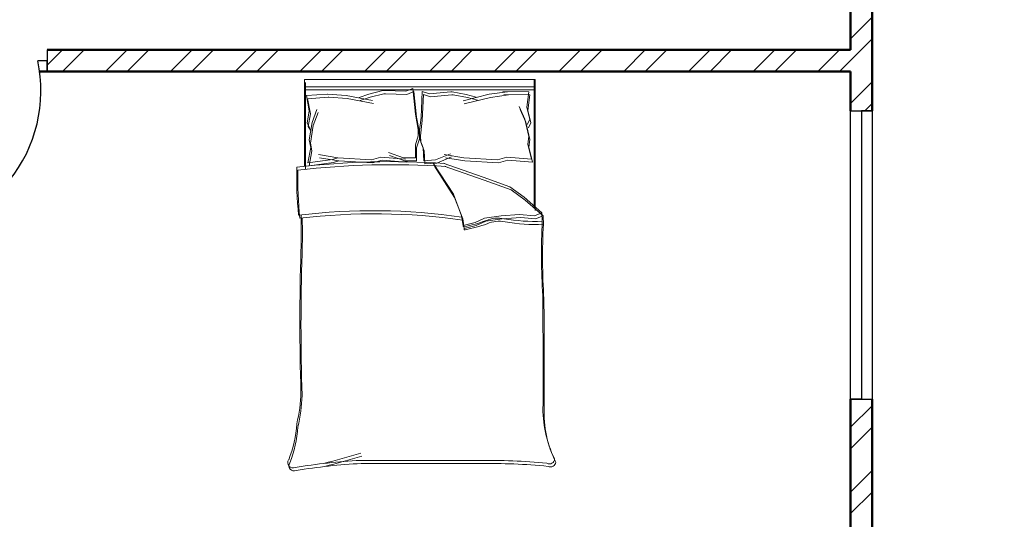
# Model space of a CAD drawing. Units: inches. Extents: x 963 to 2075, y 289 to 2657.
# Tile 88 of 98: x 1681 to 1885, y 2117 to 2221. Entities that reach past the tile are written whole.
import ezdxf

# ---------------------------------------------------------------- set-up
doc = ezdxf.new("R2010")
doc.units = ezdxf.units.IN
for name, color, linetype, lineweight in [('A-DOOR', 4, 'Continuous', 25), ('A-FURN', 8, 'Continuous', 18), ('A-GLAZ', 3, 'Continuous', 25), ('A-WALL', 7, 'Continuous', 50), ('A-WALL-PATT', 8, 'Continuous', 13)]:
    doc.layers.add(name, color=color, linetype=linetype, lineweight=lineweight)

# ---------------------------------------------------------------- blocks, each defined once
blk = doc.blocks.new('BED-DOUBLE')
for p, q in [((1236.12, 2450.52), (1254.23, 2450.52)), ((1236.12, 2450.52), (1254.23, 2450.52)), ((1236.76, 2450.75), (1254.87, 2450.75)), ((1236.76, 2450.75), (1254.87, 2450.75)), ((1237.61, 2444.71), (1236.89, 2449.81)), ((1236.89, 2449.81), (1240.07, 2449.23)), ((1237.61, 2444.71), (1236.89, 2449.81)), ((1236.89, 2449.81), (1240.07, 2449.23)), ((1238.25, 2444.94), (1237.53, 2450.04)), ((1237.53, 2450.04), (1240.71, 2449.46)), ((1238.25, 2444.94), (1237.53, 2450.04)), ((1237.53, 2450.04), (1240.71, 2449.46)), ((1245.13, 2449.96), (1244.12, 2449.38)), ((1245.13, 2449.96), (1244.12, 2449.38)), ((1245.77, 2450.18), (1244.76, 2449.61)), ((1245.77, 2450.18), (1244.76, 2449.61)), ((1247.74, 2449.52), (1245.13, 2449.96)), ((1247.74, 2449.52), (1245.13, 2449.96)), ((1248.37, 2449.75), (1245.77, 2450.18)), ((1248.37, 2449.75), (1245.77, 2450.18)), ((1250.92, 2450.1), (1247.74, 2449.52)), ((1250.92, 2450.1), (1247.74, 2449.52)), ((1251.56, 2450.33), (1248.37, 2449.75)), ((1251.56, 2450.33), (1248.37, 2449.75)), ((1250.89, 2450.1), (1251.22, 2445.82)), ((1250.89, 2450.1), (1251.22, 2445.82)), ((1251.53, 2450.32), (1251.86, 2446.04)), ((1251.53, 2450.32), (1251.86, 2446.04)), ((1252.7, 2450.52), (1252.7, 2402.73)), ((1252.7, 2450.52), (1252.7, 2402.73)), ((1253.34, 2450.75), (1253.34, 2402.96)), ((1253.34, 2450.75), (1253.34, 2402.96)), ((1254.87, 2450.75), (1254.87, 2402.73)), ((1239.24, 2447.84), (1238.58, 2443.81)), ((1239.24, 2447.84), (1238.58, 2443.81)), ((1240.07, 2449.23), (1241.66, 2449.52)), ((1240.07, 2449.23), (1241.66, 2449.52)), ((1240.71, 2449.46), (1242.3, 2449.75)), ((1240.71, 2449.46), (1242.3, 2449.75)), ((1241.66, 2449.52), (1245.28, 2448.94)), ((1241.66, 2449.52), (1245.28, 2448.94)), ((1242.3, 2449.75), (1245.92, 2449.17)), ((1242.3, 2449.75), (1245.92, 2449.17)), ((1245.28, 2448.94), (1248.02, 2447.93)), ((1245.28, 2448.94), (1248.02, 2447.93)), ((1245.92, 2449.17), (1248.66, 2448.16)), ((1245.92, 2449.17), (1248.66, 2448.16)), ((1238.6, 2447.61), (1237.94, 2443.58)), ((1238.6, 2447.61), (1237.94, 2443.58)), ((1251.21, 2445.71), (1250.92, 2441.89)), ((1251.21, 2445.71), (1250.92, 2441.89)), ((1251.22, 2445.82), (1251.21, 2445.71)), ((1251.22, 2445.82), (1251.21, 2445.71)), ((1251.84, 2445.94), (1251.56, 2442.11)), ((1251.84, 2445.94), (1251.56, 2442.11)), ((1251.86, 2446.04), (1251.84, 2445.94)), ((1251.86, 2446.04), (1251.84, 2445.94)), ((1237.94, 2443.58), (1237.61, 2444.71)), ((1237.94, 2443.58), (1237.61, 2444.71)), ((1238.58, 2443.81), (1238.15, 2436.8)), ((1238.58, 2443.81), (1238.15, 2436.8)), ((1238.58, 2443.81), (1238.25, 2444.94)), ((1238.58, 2443.81), (1238.25, 2444.94)), ((1237.94, 2443.58), (1237.51, 2436.57)), ((1237.94, 2443.58), (1237.51, 2436.57)), ((1250.92, 2441.89), (1249.9, 2436.39)), ((1250.92, 2441.89), (1249.9, 2436.39)), ((1251.56, 2442.11), (1250.54, 2436.62)), ((1251.56, 2442.11), (1250.54, 2436.62)), ((1174.99, 2438.93), (1174.99, 2414.32)), ((1174.99, 2438.93), (1174.99, 2414.32)), ((1175.63, 2439.16), (1175.63, 2414.55)), ((1175.63, 2439.16), (1175.63, 2414.55)), ((1250.48, 2439.14), (1251.21, 2437.12)), ((1250.48, 2439.14), (1251.21, 2437.12)), ((1251.12, 2439.37), (1251.84, 2437.34)), ((1251.12, 2439.37), (1251.84, 2437.34)), ((1237.51, 2436.57), (1238.06, 2434.61)), ((1237.51, 2436.57), (1238.06, 2434.61)), ((1238.15, 2436.8), (1238.7, 2434.84)), ((1238.15, 2436.8), (1238.7, 2434.84)), ((1251.21, 2437.12), (1251.93, 2434.22)), ((1251.21, 2437.12), (1251.93, 2434.23)), ((1251.84, 2437.34), (1252.57, 2434.45)), ((1251.84, 2437.34), (1252.57, 2434.45)), ((1238.06, 2434.61), (1237.66, 2429.48)), ((1238.06, 2434.61), (1237.66, 2429.48)), ((1238.7, 2434.84), (1238.3, 2429.71)), ((1238.7, 2434.84), (1238.3, 2429.71)), ((1251.93, 2433.9), (1251.78, 2429.46)), ((1251.93, 2433.9), (1251.78, 2429.46)), ((1251.93, 2434.23), (1251.93, 2433.9)), ((1251.93, 2434.22), (1251.93, 2433.9)), ((1252.57, 2434.13), (1252.42, 2429.69)), ((1252.57, 2434.13), (1252.42, 2429.69)), ((1252.57, 2434.45), (1252.57, 2434.13)), ((1252.57, 2434.45), (1252.57, 2434.13)), ((1237.97, 2429.89), (1239.06, 2433.04)), ((1237.97, 2429.89), (1239.06, 2433.04)), ((1238.61, 2430.12), (1239.7, 2433.26)), ((1238.61, 2430.12), (1239.7, 2433.26)), ((1237.97, 2427.43), (1237.97, 2429.89)), ((1237.97, 2427.43), (1237.97, 2429.89)), ((1238.61, 2427.66), (1238.61, 2430.12)), ((1238.61, 2427.66), (1238.61, 2430.12)), ((1251.78, 2429.46), (1252.36, 2428.01)), ((1251.78, 2429.46), (1252.36, 2428.01)), ((1252.42, 2429.69), (1253, 2428.24)), ((1252.42, 2429.69), (1253, 2428.24)), ((1240.65, 2427.43), (1237.97, 2427.43)), ((1240.65, 2427.43), (1237.97, 2427.43)), ((1241.29, 2427.66), (1238.61, 2427.66)), ((1241.29, 2427.66), (1238.61, 2427.66)), ((1242.53, 2426.86), (1240.65, 2427.43)), ((1242.53, 2426.86), (1240.65, 2427.43)), ((1243.17, 2427.08), (1241.29, 2427.66)), ((1243.17, 2427.08), (1241.29, 2427.66)), ((1247.01, 2427.43), (1243.83, 2426.86)), ((1247.01, 2427.43), (1243.83, 2426.86)), ((1247.65, 2427.66), (1244.47, 2427.08)), ((1247.65, 2427.66), (1244.47, 2427.08)), ((1252.36, 2428.01), (1247.01, 2427.43)), ((1252.36, 2428.01), (1247.01, 2427.43)), ((1253, 2428.24), (1247.65, 2427.66)), ((1253, 2428.24), (1247.65, 2427.66)), ((1240.02, 2425.86), (1237.34, 2425.7)), ((1240.02, 2425.86), (1237.34, 2425.7)), ((1237.34, 2425.7), (1237.49, 2423.24)), ((1237.34, 2425.7), (1237.49, 2423.24)), ((1240.66, 2426.09), (1237.98, 2425.93)), ((1240.66, 2426.09), (1237.98, 2425.93)), ((1237.98, 2425.93), (1238.13, 2423.47)), ((1237.98, 2425.93), (1238.13, 2423.47)), ((1241.86, 2426.56), (1240.02, 2425.86)), ((1241.86, 2426.56), (1240.02, 2425.86)), ((1242.49, 2426.79), (1240.66, 2426.09)), ((1242.49, 2426.79), (1240.66, 2426.09)), ((1243.15, 2426.64), (1241.86, 2426.56)), ((1243.15, 2426.64), (1241.86, 2426.56)), ((1243.79, 2426.87), (1242.49, 2426.79)), ((1243.79, 2426.87), (1242.49, 2426.79)), ((1243.83, 2426.86), (1242.53, 2426.86)), ((1243.83, 2426.86), (1242.53, 2426.86)), ((1246.37, 2426.26), (1243.15, 2426.64)), ((1246.37, 2426.26), (1243.15, 2426.64)), ((1244.47, 2427.08), (1243.17, 2427.08)), ((1244.47, 2427.08), (1243.17, 2427.08)), ((1247, 2426.49), (1243.79, 2426.87)), ((1247, 2426.49), (1243.79, 2426.87)), ((1251.74, 2426.02), (1246.37, 2426.26)), ((1251.74, 2426.02), (1246.37, 2426.26)), ((1252.38, 2426.25), (1247, 2426.49)), ((1252.38, 2426.25), (1247, 2426.49)), ((1251.25, 2424.54), (1251.74, 2426.02)), ((1251.25, 2424.54), (1251.74, 2426.02)), ((1251.89, 2424.77), (1252.38, 2426.25)), ((1251.89, 2424.77), (1252.38, 2426.25)), ((1236.85, 2423.74), (1230.36, 2419.55)), ((1236.85, 2423.74), (1230.36, 2419.55)), ((1237.49, 2423.96), (1231, 2419.77)), ((1237.49, 2423.96), (1231, 2419.77)), ((1237.49, 2423.24), (1238.78, 2420.17)), ((1237.49, 2423.24), (1238.78, 2420.17)), ((1238.13, 2423.47), (1239.42, 2420.4)), ((1238.13, 2423.47), (1239.42, 2420.4)), ((1251.68, 2420.11), (1251.25, 2424.54)), ((1251.68, 2420.11), (1251.25, 2424.54)), ((1252.31, 2420.34), (1251.89, 2424.77)), ((1252.31, 2420.34), (1251.89, 2424.77)), ((1233.92, 2413.35), (1236.85, 2421.69)), ((1233.92, 2413.35), (1236.85, 2421.69)), ((1234.56, 2413.58), (1237.49, 2421.92)), ((1234.56, 2413.58), (1237.49, 2421.92)), ((1238.6, 2421.43), (1237.94, 2417.4)), ((1238.6, 2421.43), (1237.94, 2417.4)), ((1239.24, 2421.66), (1238.58, 2417.63)), ((1239.24, 2421.66), (1238.58, 2417.63)), ((1230.36, 2419.55), (1225.87, 2417.84)), ((1230.36, 2419.55), (1225.87, 2417.84)), ((1231, 2419.77), (1226.51, 2418.07)), ((1231, 2419.77), (1226.51, 2418.07)), ((1251.15, 2416.86), (1251.7, 2419.79)), ((1251.15, 2416.86), (1251.7, 2419.79)), ((1251.7, 2419.79), (1251.68, 2420.11)), ((1251.7, 2419.79), (1251.68, 2420.11)), ((1251.79, 2417.09), (1252.33, 2420.02)), ((1251.79, 2417.09), (1252.33, 2420.02)), ((1252.33, 2420.02), (1252.31, 2420.34)), ((1252.33, 2420.02), (1252.31, 2420.34)), ((1225.87, 2417.84), (1223.86, 2417.53)), ((1225.87, 2417.84), (1223.86, 2417.53)), ((1223.86, 2417.53), (1224.47, 2415.05)), ((1223.86, 2417.53), (1224.47, 2415.05)), ((1226.51, 2418.07), (1224.49, 2417.76)), ((1226.51, 2418.07), (1224.49, 2417.76)), ((1224.49, 2417.76), (1225.11, 2415.28)), ((1224.49, 2417.76), (1225.11, 2415.28)), ((1237.94, 2417.4), (1237.51, 2410.39)), ((1237.94, 2417.4), (1237.51, 2410.39)), ((1238.58, 2417.63), (1238.15, 2410.62)), ((1238.58, 2417.63), (1238.15, 2410.62)), ((1251.16, 2412.08), (1249.81, 2417.5)), ((1251.16, 2412.08), (1249.81, 2417.5)), ((1251.8, 2412.31), (1250.45, 2417.73)), ((1251.8, 2412.31), (1250.45, 2417.73)), ((1251.2, 2415.02), (1251.79, 2417.09)), ((1251.2, 2415.02), (1251.79, 2417.09)), ((1224.47, 2415.05), (1225.4, 2413.04)), ((1224.47, 2415.05), (1225.4, 2413.04)), ((1225.11, 2415.28), (1226.04, 2413.27)), ((1225.11, 2415.28), (1226.04, 2413.27)), ((1250.56, 2414.79), (1251.15, 2416.86)), ((1250.56, 2414.79), (1251.15, 2416.86)), ((1225.4, 2413.04), (1225.87, 2409.63)), ((1225.4, 2413.04), (1225.87, 2409.63)), ((1226.04, 2413.27), (1226.51, 2409.86)), ((1226.04, 2413.27), (1226.51, 2409.86)), ((1231.9, 2407.77), (1233.92, 2413.35)), ((1231.9, 2407.78), (1233.92, 2413.35)), ((1232.54, 2408), (1234.56, 2413.58)), ((1232.54, 2408), (1234.56, 2413.58)), ((1251.69, 2408.28), (1251.16, 2412.08)), ((1251.69, 2408.28), (1251.16, 2412.08)), ((1252.33, 2408.51), (1251.8, 2412.31)), ((1252.33, 2408.51), (1251.8, 2412.31)), ((1225.87, 2409.63), (1226.18, 2405.76)), ((1225.87, 2409.63), (1226.18, 2405.76)), ((1226.51, 2409.86), (1226.82, 2405.99)), ((1226.51, 2409.86), (1226.82, 2405.99)), ((1237.51, 2410.39), (1238.06, 2408.43)), ((1237.51, 2410.39), (1238.06, 2408.43)), ((1238.15, 2410.62), (1238.7, 2408.66)), ((1238.15, 2410.62), (1238.7, 2408.66)), ((1251.68, 2403.88), (1251.77, 2409.29)), ((1251.68, 2403.88), (1251.77, 2409.28)), ((1251.77, 2409.29), (1251.69, 2408.28)), ((1251.77, 2409.28), (1251.69, 2408.28)), ((1252.31, 2404.11), (1252.41, 2409.51)), ((1252.31, 2404.11), (1252.41, 2409.51)), ((1252.41, 2409.51), (1252.33, 2408.51)), ((1252.41, 2409.51), (1252.33, 2408.51)), ((1229.74, 2404.83), (1231.9, 2407.78)), ((1229.74, 2404.83), (1231.9, 2407.77)), ((1230.38, 2405.06), (1232.54, 2408)), ((1230.38, 2405.06), (1232.54, 2408)), ((1238.06, 2408.43), (1237.66, 2403.3)), ((1238.06, 2408.43), (1237.66, 2403.3)), ((1238.7, 2408.66), (1238.3, 2403.52)), ((1238.7, 2408.66), (1238.3, 2403.52)), ((1226.18, 2405.76), (1225.87, 2402.66)), ((1226.18, 2405.76), (1225.87, 2402.66)), ((1226.49, 2401.13), (1229.74, 2404.83)), ((1226.49, 2401.13), (1229.74, 2404.83)), ((1226.82, 2405.99), (1226.51, 2402.89)), ((1226.82, 2405.99), (1226.51, 2402.89)), ((1227.13, 2401.36), (1230.38, 2405.06)), ((1227.13, 2401.36), (1230.38, 2405.06)), ((1243.04, 2404.11), (1246.61, 2404.91)), ((1243.04, 2404.11), (1246.61, 2404.91)), ((1245.98, 2404.69), (1248.65, 2405.87)), ((1245.98, 2404.69), (1248.65, 2405.87)), ((1246.61, 2404.91), (1249.29, 2406.1)), ((1246.61, 2404.91), (1249.29, 2406.09)), ((1225.87, 2402.66), (1226.49, 2401.13)), ((1225.87, 2402.66), (1226.49, 2401.13)), ((1226.51, 2402.89), (1227.13, 2401.36)), ((1226.51, 2402.89), (1227.13, 2401.36)), ((1254.23, 2402.73), (1227.62, 2402.73)), ((1254.23, 2402.73), (1227.62, 2402.73)), ((1254.87, 2402.96), (1228.26, 2402.96)), ((1254.87, 2402.96), (1228.26, 2402.96)), ((1237.66, 2403.3), (1240.8, 2404.07)), ((1237.66, 2403.3), (1240.8, 2404.07)), ((1238.3, 2403.52), (1241.44, 2404.3)), ((1238.3, 2403.52), (1241.44, 2404.3)), ((1240.8, 2404.07), (1242.4, 2403.88)), ((1240.8, 2404.07), (1242.4, 2403.88)), ((1241.44, 2404.3), (1243.04, 2404.11)), ((1241.44, 2404.3), (1243.04, 2404.11)), ((1242.4, 2403.88), (1245.98, 2404.69)), ((1242.4, 2403.88), (1245.98, 2404.69)), ((1245.89, 2403.67), (1244.85, 2404.18)), ((1245.89, 2403.67), (1244.85, 2404.18)), ((1246.53, 2403.89), (1245.49, 2404.41)), ((1246.53, 2403.89), (1245.49, 2404.41)), ((1248.46, 2404.26), (1245.89, 2403.67)), ((1248.46, 2404.26), (1245.89, 2403.67)), ((1249.1, 2404.49), (1246.53, 2403.89)), ((1249.1, 2404.49), (1246.53, 2403.89)), ((1251.68, 2403.88), (1248.46, 2404.26)), ((1251.68, 2403.88), (1248.46, 2404.26)), ((1252.31, 2404.11), (1249.1, 2404.49)), ((1252.31, 2404.11), (1249.1, 2404.49)), ((1254.87, 2402.73), (1254.23, 2402.73)), ((1224.74, 2401.05), (1226.49, 2401.13, 3.87)), ((1224.74, 2401.05), (1226.49, 2401.13, 3.87)), ((1225.38, 2401.28), (1227.13, 2401.36, 3.87)), ((1225.38, 2401.28), (1227.13, 2401.36, 3.87))]:
    blk.add_line(p, q)
for centre, radius, start, end in [((1174.51, 2452.91), 1.09, 56.1736, 203.4781), ((1174.51, 2452.91), 1.09, 56.1736, 203.4781), ((1175.15, 2453.14), 1.09, 56.1736, 203.4781), ((1175.15, 2453.14), 1.09, 56.1736, 203.4781), ((1184.6, 2475.88), 23.56, 247.9751, 266.652), ((1184.6, 2475.88), 23.56, 247.9751, 266.652), ((1053.4, 2432.57), 121.76, 2.9958, 9.4091), ((1053.4, 2432.57), 121.76, 2.9958, 9.4091), ((1054.03, 2432.8), 121.76, 2.9958, 9.4091), ((1054.03, 2432.8), 121.76, 2.9958, 9.4091), ((1183.96, 2475.65), 23.56, 247.9751, 266.652), ((1183.96, 2475.65), 23.56, 247.9751, 266.652), ((1189.72, 2480.89), 29.63, 256.0648, 268.9113), ((1189.72, 2480.89), 29.63, 256.0648, 268.9113), ((1190.36, 2481.12), 29.63, 256.0648, 268.9113), ((1190.36, 2481.12), 29.63, 256.0648, 268.9113), ((1234.14, 2368.83), 83.31, 88.7218, 95.604), ((1234.14, 2368.83), 83.31, 88.7218, 95.604), ((1098.56, 2436.47), 129.02, 351.7845, 6.9006), ((1098.56, 2436.47), 129.02, 351.7845, 6.9006), ((1234.78, 2369.06), 83.31, 88.7218, 95.604), ((1234.78, 2369.06), 83.31, 88.7218, 95.604), ((1072.18, 2432.64), 164.97, 356.0865, 6.7821), ((1072.18, 2432.64), 164.97, 356.0865, 6.7821), ((1072.82, 2432.86), 164.97, 356.0865, 6.7821), ((1072.82, 2432.86), 164.97, 356.0865, 6.7821), ((1203.62, 1969.17), 482.31, 88.2277, 91.7185), ((1203.62, 1969.17), 482.31, 88.2277, 91.7185), ((1204.26, 1969.4), 482.31, 88.2277, 91.7185), ((1204.26, 1969.4), 482.31, 88.2277, 91.7185), ((1223.06, 2621.3), 170.11, 268.4762, 271.0082), ((1223.06, 2621.3), 170.11, 268.4762, 271.0082), ((1223.7, 2621.53), 170.11, 268.4762, 271.0082), ((1223.7, 2621.53), 170.11, 268.4762, 271.0082), ((1097.92, 2436.24), 129.02, 351.7845, 6.9006), ((1097.92, 2436.24), 129.02, 351.7845, 6.9006), ((1277.94, 2471.22), 106.46, 193.3832, 197.7053), ((1277.94, 2471.22), 106.46, 193.3832, 197.7053), ((1278.58, 2471.44), 106.46, 193.3832, 197.7053), ((1278.58, 2471.44), 106.46, 193.3832, 197.7053), ((1223.79, 2417.36), 0.185, 70.2464, 181.1377), ((1223.79, 2417.36), 0.185, 70.2464, 181.1377), ((1252.75, 2422.84), 29.65, 190.6617, 199.8806), ((1252.75, 2422.84), 29.65, 190.6617, 199.8806), ((1224.43, 2417.59), 0.185, 70.2464, 181.1377), ((1224.43, 2417.59), 0.185, 70.2464, 181.1377), ((1253.39, 2423.07), 29.65, 190.6617, 199.8806), ((1253.39, 2423.07), 29.65, 190.6617, 199.8806), ((1041.96, 2412.84), 133.04, 354.4998, 0.6351), ((1041.96, 2412.84), 133.04, 354.4998, 0.6351), ((1042.6, 2413.07), 133.04, 354.4998, 0.6351), ((1042.6, 2413.07), 133.04, 354.4998, 0.6351), ((1219.81, 2410.48), 6.22, 348.6608, 23.7384), ((1219.81, 2410.48), 6.22, 348.6608, 23.7384), ((1219.17, 2410.25), 6.22, 348.6608, 23.7384), ((1219.17, 2410.25), 6.22, 348.6608, 23.7384), ((1260.89, 2402.67), 36.18, 169.8763, 182.5657), ((1260.89, 2402.67), 36.18, 169.8763, 182.5657), ((1261.53, 2402.9), 36.18, 169.8763, 182.5657), ((1261.53, 2402.9), 36.18, 169.8763, 182.5657), ((1185.57, 2377.84), 23.07, 87.4714, 116.4681), ((1185.57, 2377.84), 23.07, 87.4714, 116.4681), ((1186.21, 2378.07), 23.07, 87.4714, 116.4681), ((1186.21, 2378.07), 23.07, 87.4714, 116.4681), ((1186.41, 6962.74), 4561.86, 270.00217, 270.28689), ((1186.41, 6962.74), 4561.86, 270.00217, 270.28689), ((1187.05, 6962.97), 4561.86, 270.00217, 270.28689), ((1187.05, 6962.97), 4561.86, 270.00217, 270.28689), ((1217.92, 2271.73), 129.5, 86.9791, 93.8365), ((1217.92, 2271.73), 129.5, 86.9791, 93.8365), ((1218.56, 2271.96), 129.5, 86.9791, 93.8365), ((1218.56, 2271.96), 129.5, 86.9791, 93.8365), ((1175.36, 2399.58), 1.1, 152.6588, 266.02), ((1175.36, 2399.58), 1.1, 152.6588, 266.02), ((1176, 2399.81), 1.1, 152.6588, 266.02), ((1176, 2399.81), 1.1, 152.6588, 266.02)]:
    blk.add_arc(centre, radius, start, end)

msp = doc.modelspace()

# ---------------------------------------------------------------- hatches: boundary and pattern name
at = {"layer": 'A-WALL-PATT'}
h = msp.add_hatch(dxfattribs=at)
h.set_pattern_fill('ANSI32', color=256)
h.paths.add_polyline_path([(1296.92, 2558.32), (1203.92, 2558.32), (1203.92, 2493.82), (1191.53, 2493.82), (1191.53, 2489.32), (1211.06, 2489.32), (1211.06, 2492.02), (1211.06, 2493.82), (1208.42, 2493.82), (1208.42, 2553.82), (1292.42, 2553.82), (1292.42, 2538.86), (1296.92, 2538.86)])
h.paths.add_polyline_path([(1442.42, 2558.32), (1349.42, 2558.32), (1349.42, 2538.94), (1353.92, 2538.94), (1353.92, 2553.82), (1437.92, 2553.82), (1437.92, 2493.82), (1434.54, 2493.82), (1434.54, 2489.32), (1448.31, 2489.32), (1448.31, 2491.57), (1448.31, 2493.82), (1442.42, 2493.82)])
h.paths.add_polyline_path([(1415.55, 2491.57), (1415.55, 2493.82), (1340.94, 2493.82), (1340.94, 2489.32), (1371.92, 2489.32), (1371.92, 2378.32), (1367.6, 2378.32), (1367.6, 2373.82), (1371.92, 2373.82), (1371.92, 2355.19), (1376.42, 2355.19), (1376.42, 2489.32), (1415.55, 2489.32)])
h.paths.add_polyline_path([(1304.94, 2491.57), (1304.94, 2493.82), (1296.92, 2493.82), (1296.92, 2514.86), (1292.42, 2514.86), (1292.42, 2493.82), (1232.81, 2493.82), (1232.81, 2489.32), (1256.42, 2489.32), (1256.42, 2327.32), (1253.71, 2327.32), (1253.71, 2322.82), (1328.42, 2322.82), (1328.42, 2331.15), (1323.92, 2331.15), (1323.92, 2327.32), (1260.92, 2327.32), (1260.92, 2373.82), (1323.92, 2373.82), (1323.92, 2357.81), (1328.42, 2357.81), (1328.42, 2373.82), (1346.01, 2373.82), (1346.01, 2376.07), (1346.01, 2378.32), (1260.92, 2378.32), (1260.92, 2489.32), (1304.94, 2489.32)])
h.paths.add_polyline_path([(1226.65, 2327.32), (1124.42, 2327.32), (1124.42, 2347.45), (1119.92, 2347.45), (1119.92, 2322.82), (1163.42, 2322.82), (1163.42, 2305.43), (1165.67, 2305.43), (1167.92, 2305.43), (1167.92, 2322.82), (1226.65, 2322.82), (1226.65, 2325.07)])
h.paths.add_polyline_path([(1095.92, 2489.32), (1124.42, 2489.32), (1131.53, 2489.32), (1131.53, 2491.57), (1131.53, 2493.82), (1119.92, 2493.82), (1091.42, 2493.82), (1091.42, 2417.32), (1095.92, 2417.32), (1119.92, 2417.32), (1119.92, 2407.45), (1124.42, 2407.45), (1124.42, 2421.82), (1095.92, 2421.82)])
h.paths.add_polyline_path([(1512.92, 2558.32), (1508.42, 2558.32), (1508.42, 2493.82), (1503.4, 2493.82), (1503.4, 2489.32), (1508.42, 2489.32), (1508.42, 2327.32), (1376.42, 2327.32), (1376.42, 2330.27), (1371.92, 2330.27), (1371.92, 2298.74), (1376.42, 2298.74), (1376.42, 2322.82), (1508.42, 2322.82), (1508.42, 2165.32), (1504.26, 2165.32), (1504.26, 2160.82), (1508.42, 2160.82), (1508.42, 2108.32), (1512.92, 2108.32), (1512.92, 2160.82), (1516.18, 2160.82), (1516.18, 2163.07), (1516.18, 2165.32), (1512.92, 2165.32), (1512.92, 2322.82), (1644.92, 2322.82), (1644.92, 2298.74), (1649.42, 2298.74), (1649.42, 2322.82), (1649.42, 2330.94), (1647.17, 2330.94), (1644.92, 2330.94), (1644.92, 2327.32), (1512.92, 2327.32), (1512.92, 2489.32), (1516.76, 2489.32), (1516.76, 2491.57), (1516.76, 2493.82), (1512.92, 2493.82)])
h.paths.add_polyline_path([(1671.92, 2558.32), (1578.92, 2558.32), (1578.92, 2493.82), (1573.53, 2493.82), (1573.53, 2489.32), (1586.54, 2489.32), (1586.54, 2491.57), (1586.54, 2493.82), (1583.42, 2493.82), (1583.42, 2553.82), (1667.42, 2553.82), (1667.42, 2541.11), (1671.92, 2541.11)])
h.paths.add_polyline_path([(1681.26, 2493.82), (1671.92, 2493.82), (1671.92, 2517.11), (1667.42, 2517.11), (1667.42, 2493.82), (1610.22, 2493.82), (1610.22, 2489.32), (1644.92, 2489.32), (1644.92, 2357.87), (1649.42, 2357.87), (1649.42, 2373.82), (1652.2, 2373.82), (1652.2, 2375.83), (1652.2, 2378.32), (1649.42, 2378.32), (1649.42, 2489.32), (1681.26, 2489.32), (1681.26, 2491.57)])
h.paths.add_polyline_path([(1821.92, 2558.32), (1728.92, 2558.32), (1728.92, 2541), (1733.42, 2541), (1733.42, 2553.82), (1817.42, 2553.82), (1817.42, 2493.82), (1813.51, 2493.82), (1813.51, 2489.32), (1830.08, 2489.32), (1830.08, 2491.57), (1830.08, 2493.82), (1821.92, 2493.82)])
h.paths.add_polyline_path([(1794.24, 2493.82), (1717.26, 2493.82), (1717.26, 2489.32), (1760.42, 2489.32), (1760.42, 2378.32), (1674.4, 2378.32), (1674.4, 2373.82), (1692.92, 2373.82), (1692.92, 2356.95), (1697.42, 2356.95), (1697.42, 2373.82), (1760.42, 2373.82), (1760.42, 2327.32), (1697.42, 2327.32), (1697.42, 2333.34), (1692.92, 2333.34), (1692.92, 2322.82), (1768.04, 2322.82), (1768.04, 2325.07), (1768.04, 2327.32), (1764.92, 2327.32), (1764.92, 2489.32), (1794.24, 2489.32)])
h.paths.add_polyline_path([(1733.42, 2517), (1728.92, 2517), (1728.92, 2493.82), (1733.42, 2493.82)], flags=17)
h.paths.add_polyline_path([(1929.92, 2493.82), (1890.08, 2493.82), (1890.08, 2489.32), (1896.92, 2489.32), (1925.42, 2489.32), (1925.42, 2421.82), (1896.92, 2421.82), (1896.92, 2408.32), (1901.42, 2408.32), (1901.42, 2417.32), (1925.42, 2417.32), (1929.92, 2417.32)])
h.paths.add_polyline_path([(1901.42, 2348.32), (1896.92, 2348.32), (1896.92, 2327.32), (1800.42, 2327.32), (1800.42, 2322.82), (1853.42, 2322.82), (1853.42, 2309.45), (1857.92, 2309.45), (1857.92, 2322.82), (1901.42, 2322.82)])
h.paths.add_polyline_path([(1857.92, 2249.45), (1853.42, 2249.45), (1853.42, 2214.82), (1686.31, 2214.82), (1686.31, 2210.32), (1853.42, 2210.32), (1853.42, 2202.13), (1857.92, 2202.13), (1857.92, 2210.32)])
h.paths.add_polyline_path([(1857.92, 2142.13), (1853.42, 2142.13), (1853.42, 2115.42), (1841.42, 2115.42), (1841.42, 2088.53), (1841.42, 2046.95), (1845.92, 2046.95), (1845.92, 2110.92), (1905.92, 2110.92), (1905.92, 2092.52), (1910.42, 2092.52), (1910.42, 2115.42), (1857.92, 2115.42)])
h.paths.add_polyline_path([(1532.44, 1482.34), (1573.46, 1482.34), (1573.46, 1501), (1532.44, 1501)], flags=9)
h.paths.add_polyline_path([(1438.66, 1486.3), (1479.68, 1486.3), (1479.68, 1504.96), (1438.66, 1504.96)], flags=9)
h.paths.add_polyline_path([(1411.22, 1365.31), (1659.14, 1365.31), (1659.14, 1402.4), (1411.22, 1402.4)], flags=9)
h.paths.add_polyline_path([(1185.67, 2296.3), (1248.16, 2296.3), (1248.16, 2314.95), (1185.67, 2314.95)], flags=9)
h.paths.add_polyline_path([(1177.31, 2187.35), (1216.15, 2187.35), (1216.15, 2206.01), (1177.31, 2206.01)], flags=9)
h.paths.add_polyline_path([(1295.1, 1602.08), (1328.26, 1602.08), (1328.26, 1620.74), (1295.1, 1620.74)], flags=9)
h.paths.add_polyline_path([(1525.13, 2005.99), (1558.39, 2005.99), (1558.39, 2024.65), (1525.13, 2024.65)], flags=9)
h.paths.add_polyline_path([(1459.61, 1977.13), (1472.19, 1977.13), (1472.19, 1987.43), (1459.61, 1987.43)], flags=9)
h.paths.add_polyline_path([(1467.81, 2053.68), (1480.02, 2053.68), (1480.02, 2063.98), (1467.81, 2063.98)], flags=9)
h.paths.add_polyline_path([(1555.18, 2119.02), (1584.56, 2119.02), (1584.56, 2137.68), (1555.18, 2137.68)], flags=25)
h.paths.add_polyline_path([(1405.39, 2115.29), (1444.48, 2115.29), (1444.48, 2133.95), (1405.39, 2133.95)], flags=25)
h.paths.add_polyline_path([(1698.48, 2004.26), (1727.69, 2004.26), (1727.69, 2022.92), (1698.48, 2022.92)], flags=9)
h.paths.add_polyline_path([(1612.16, 1972.86), (1629.02, 1972.86), (1629.02, 1983.16), (1612.16, 1983.16)], flags=9)
h.paths.add_polyline_path([(1608.29, 2060.04), (1625.15, 2060.04), (1625.15, 2070.34), (1608.29, 2070.34)], flags=9)
h.paths.add_polyline_path([(1527.95, 1684.4), (1566.79, 1684.4), (1566.79, 1703.06), (1527.95, 1703.06)], flags=9)
h.paths.add_polyline_path([(1422.79, 1683.59), (1461.63, 1683.59), (1461.63, 1702.25), (1422.79, 1702.25)], flags=9)
h.paths.add_polyline_path([(1531.26, 1732.46), (1574.01, 1732.46), (1574.01, 1751.12), (1531.26, 1751.12)], flags=9)
h.paths.add_polyline_path([(1402.87, 1732.85), (1439.8, 1732.85), (1439.8, 1751.5), (1402.87, 1751.5)], flags=9)
h.paths.add_polyline_path([(1243.12, 1923.13), (1281.96, 1923.13), (1281.96, 1941.79), (1243.12, 1941.79)], flags=9)
h.paths.add_polyline_path([(1181.75, 1792.27), (1244.24, 1792.27), (1244.24, 1810.93), (1181.75, 1810.93)], flags=9)
h.paths.add_polyline_path([(1265.82, 1670.3), (1316.07, 1670.3), (1316.07, 1688.96), (1265.82, 1688.96)], flags=9)
h.paths.add_polyline_path([(1140.26, 1676.05), (1179.1, 1676.05), (1179.1, 1694.71), (1140.26, 1694.71)], flags=9)
h.paths.add_polyline_path([(1107.49, 1490.89), (1143.37, 1490.89), (1143.37, 1509.55), (1107.49, 1509.55)], flags=9)
h.paths.add_polyline_path([(1217.58, 1483.9), (1246.74, 1483.9), (1246.74, 1502.56), (1217.58, 1502.56)], flags=9)
h.paths.add_polyline_path([(1389.21, 1486.92), (1418.37, 1486.92), (1418.37, 1505.58), (1389.21, 1505.58)], flags=9)
h.paths.add_polyline_path([(1672.21, 1602.08), (1705.37, 1602.08), (1705.37, 1620.74), (1672.21, 1620.74)], flags=9)
h.paths.add_polyline_path([(1752.08, 1522.64), (1781.24, 1522.64), (1781.24, 1541.3), (1752.08, 1541.3)], flags=9)
h.paths.add_polyline_path([(1848.27, 1491.26), (1884.16, 1491.26), (1884.16, 1509.92), (1848.27, 1509.92)], flags=9)
h.paths.add_polyline_path([(1822.47, 1685.62), (1861.31, 1685.62), (1861.31, 1704.28), (1822.47, 1704.28)], flags=9)
h.paths.add_polyline_path([(1713.19, 1672.23), (1763.44, 1672.23), (1763.44, 1690.89), (1713.19, 1690.89)], flags=9)
h.paths.add_polyline_path([(1736.62, 1790.58), (1799.11, 1790.58), (1799.11, 1809.24), (1736.62, 1809.24)], flags=9)
h.paths.add_polyline_path([(1691.49, 1916.36), (1730.33, 1916.36), (1730.33, 1935.01), (1691.49, 1935.01)], flags=9)
h.paths.add_polyline_path([(1764.87, 1973.92), (1794.31, 1973.92), (1794.31, 1992.58), (1764.87, 1992.58)], flags=9)
h.paths.add_polyline_path([(1767.85, 2034.02), (1797.29, 2034.02), (1797.29, 2052.67), (1767.85, 2052.67)], flags=9)
h.paths.add_polyline_path([(1851.59, 2060.33), (1880.75, 2060.33), (1880.75, 2078.99), (1851.59, 2078.99)], flags=25)
h.paths.add_polyline_path([(1688.49, 2086.87), (1727.33, 2086.87), (1727.33, 2105.53), (1688.49, 2105.53)], flags=9)
h.paths.add_polyline_path([(1537.74, 2293.58), (1580.49, 2293.58), (1580.49, 2312.24), (1537.74, 2312.24)], flags=25)
h.paths.add_polyline_path([(1425.59, 2296.11), (1468.34, 2296.11), (1468.34, 2314.77), (1425.59, 2314.77)], flags=25)
h.paths.add_polyline_path([(1278.52, 2004.18), (1307.72, 2004.18), (1307.72, 2022.84), (1278.52, 2022.84)], flags=9)
h.paths.add_polyline_path([(1193.28, 1973.63), (1222.72, 1973.63), (1222.72, 1992.29), (1193.28, 1992.29)], flags=9)
h.paths.add_polyline_path([(1192.41, 2040.58), (1221.84, 2040.58), (1221.84, 2059.23), (1192.41, 2059.23)], flags=9)
h.paths.add_polyline_path([(1130.6, 1951.39), (1159.76, 1951.39), (1159.76, 1970.05), (1130.6, 1970.05)], flags=9)
h.paths.add_polyline_path([(1132.83, 2052.49), (1161.98, 2052.49), (1161.98, 2071.15), (1132.83, 2071.15)], flags=9)
h.paths.add_polyline_path([(1265.13, 2334.62), (1315.38, 2334.62), (1315.38, 2353.28), (1265.13, 2353.28)], flags=25)
h.paths.add_polyline_path([(1136.74, 2330.79), (1175.58, 2330.79), (1175.58, 2349.44), (1136.74, 2349.44)], flags=9)
h.paths.add_polyline_path([(1287.42, 2417.2), (1320.58, 2417.2), (1320.58, 2435.86), (1287.42, 2435.86)], flags=25)
h.paths.add_polyline_path([(1430.99, 2329.16), (1469.83, 2329.16), (1469.83, 2347.82), (1430.99, 2347.82)], flags=25)
h.paths.add_polyline_path([(1525.42, 2329.21), (1564.26, 2329.21), (1564.26, 2347.87), (1525.42, 2347.87)], flags=25)
h.paths.add_polyline_path([(1684.52, 2382.8), (1717.68, 2382.8), (1717.68, 2401.46), (1684.52, 2401.46)], flags=25)
h.paths.add_polyline_path([(1704.81, 2340.29), (1755.05, 2340.29), (1755.05, 2358.95), (1704.81, 2358.95)], flags=25)
h.paths.add_polyline_path([(1694.11, 2287.76), (1756.6, 2287.76), (1756.6, 2306.41), (1694.11, 2306.41)], flags=9)
h.paths.add_polyline_path([(1815.78, 2329.86), (1854.62, 2329.86), (1854.62, 2348.52), (1815.78, 2348.52)], flags=9)
h.paths.add_polyline_path([(1842.87, 2514.26), (1878.76, 2514.26), (1878.76, 2532.91), (1842.87, 2532.91)], flags=9)
h.paths.add_polyline_path([(1769.51, 2531.45), (1798.67, 2531.45), (1798.67, 2550.1), (1769.51, 2550.1)], flags=25)
h.paths.add_polyline_path([(1594.77, 2518.47), (1623.93, 2518.47), (1623.93, 2537.13), (1594.77, 2537.13)], flags=25)
h.paths.add_polyline_path([(1520.72, 2516.18), (1556.61, 2516.18), (1556.61, 2534.84), (1520.72, 2534.84)], flags=25)
h.paths.add_polyline_path([(1464.46, 2516.69), (1500.34, 2516.69), (1500.34, 2535.35), (1464.46, 2535.35)], flags=25)
h.paths.add_polyline_path([(1365.7, 2528.97), (1394.85, 2528.97), (1394.85, 2547.63), (1365.7, 2547.63)], flags=25)
h.paths.add_polyline_path([(1222.84, 2516.23), (1252, 2516.23), (1252, 2534.89), (1222.84, 2534.89)], flags=25)
h.paths.add_polyline_path([(1104.55, 2509.6), (1140.43, 2509.6), (1140.43, 2528.26), (1104.55, 2528.26)], flags=9)

# ---------------------------------------------------------------- linework, layer by layer
at = {"layer": 'A-DOOR'}
for p, q in [((1686.31, 2214.82), (1686.31, 2210.32)), ((1686.31, 2212.57), (1684.31, 2212.57)), ((1686.31, 2210.32), (1686.31, 2212.57))]:
    msp.add_line(p, q, dxfattribs=at)
msp.add_arc((1655.23, 2206.32), 29.75, 270, 12.1318, dxfattribs=at)
at = {"layer": 'A-GLAZ'}
for p, q in [((1853.42, 2202.13), (1857.92, 2202.13)), ((1853.42, 2142.13), (1853.42, 2202.13)), ((1857.92, 2202.13), (1855.67, 2202.13)), ((1855.67, 2202.13), (1855.67, 2142.13)), ((1857.92, 2202.13), (1857.92, 2142.13)), ((1855.67, 2142.13), (1853.42, 2142.13)), ((1853.42, 2142.13), (1857.92, 2142.13))]:
    msp.add_line(p, q, dxfattribs=at)
at = {"layer": 'A-WALL'}
for p, q in [((1853.42, 2249.45), (1853.42, 2214.82)), ((1857.92, 2249.45), (1857.92, 2210.32)), ((1686.31, 2214.82), (1853.42, 2214.82)), ((1684.7, 2210.32), (1853.42, 2210.32)), ((1853.42, 2210.32), (1853.42, 2202.13)), ((1857.92, 2202.13), (1857.92, 2210.32)), ((1853.42, 2142.13), (1853.42, 2115.42)), ((1857.92, 2115.42), (1857.92, 2142.13))]:
    msp.add_line(p, q, dxfattribs=at)

# ---------------------------------------------------------------- block references
at = {"layer": 'A-FURN', "rotation": 89.99999983318565}
msp.add_blockref('BED-DOUBLE', (4190.56, 953.79), dxfattribs=at)

doc.saveas('drawing.dxf')
